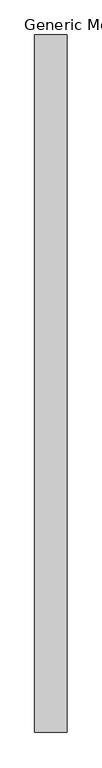
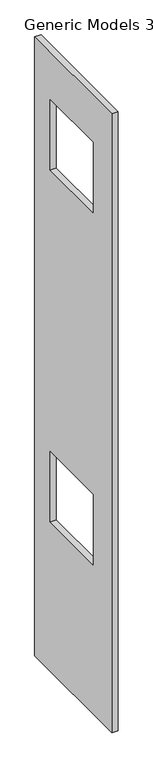
"""IFC4 building model written with IfcOpenShell, lengths in millimetres: proxy geometry, Generic Models 3 : Generic Models 3."""

from ifc_helpers import new_model, si_unit, frame, origin, place, context, project, spatial, polyline, outline, extrude, source, transform, mapped, element, save


def generic_models_3_generic_models_3_c18588e6(model_context):
    return source(origin(), model_context, "Body", "SweptSolid", [
        extrude(outline(polyline([(8788.4641252, 9369.0165262), (8788.4641252, 4007.4200537), (7693.523046, 4007.4200537), (7693.523046, 9369.0165262), (8788.4641252, 9369.0165262)]), holes=[polyline([(8572.5641252, 8956.2819261), (7962.9641252, 8956.2819261), (7962.9641252, 8346.6819261), (8572.5641252, 8346.6819261), (8572.5641252, 8956.2819261)]), polyline([(8572.5641252, 5908.2819261), (7962.9641252, 5908.2819261), (7962.9641252, 5298.6819261), (8572.5641252, 5298.6819261), (8572.5641252, 5908.2819261)])]), frame((4189.5719693, 0.0, 0.0), z_axis=(1.0, 0.0, 0.0), x_axis=(0.0, 1.0, 0.0)), (0.0, 0.0, 1.0), 50.8),
    ])


if __name__ == "__main__":
    model = new_model("IFC4")
    model_context = context("Model", 3, world=origin())
    ifc_project = project(units=[si_unit("LENGTHUNIT", "METRE", prefix="MILLI")], contexts=[model_context])
    site = spatial("IfcSite", under=ifc_project)
    building = spatial("IfcBuilding", under=site)
    placement = place(None, origin())
    generic_models_3_generic_models_3_shape = generic_models_3_generic_models_3_c18588e6(model_context)
    element("IfcBuildingElementProxy", 1, Name="Generic Models 3 : Generic Models 3", ObjectType="Generic Models 3 : Generic Models 3", at=placement, inside=building, context=model_context, shape_type="MappedRepresentation", body=[
        mapped(generic_models_3_generic_models_3_shape, transform((0.0, 0.0, 0.0), x_axis=(1.0, 0.0, 0.0), y_axis=(0.0, 1.0, 0.0), z_axis=(0.0, 0.0, 1.0))),
    ])
    save(model, "model.ifc")
